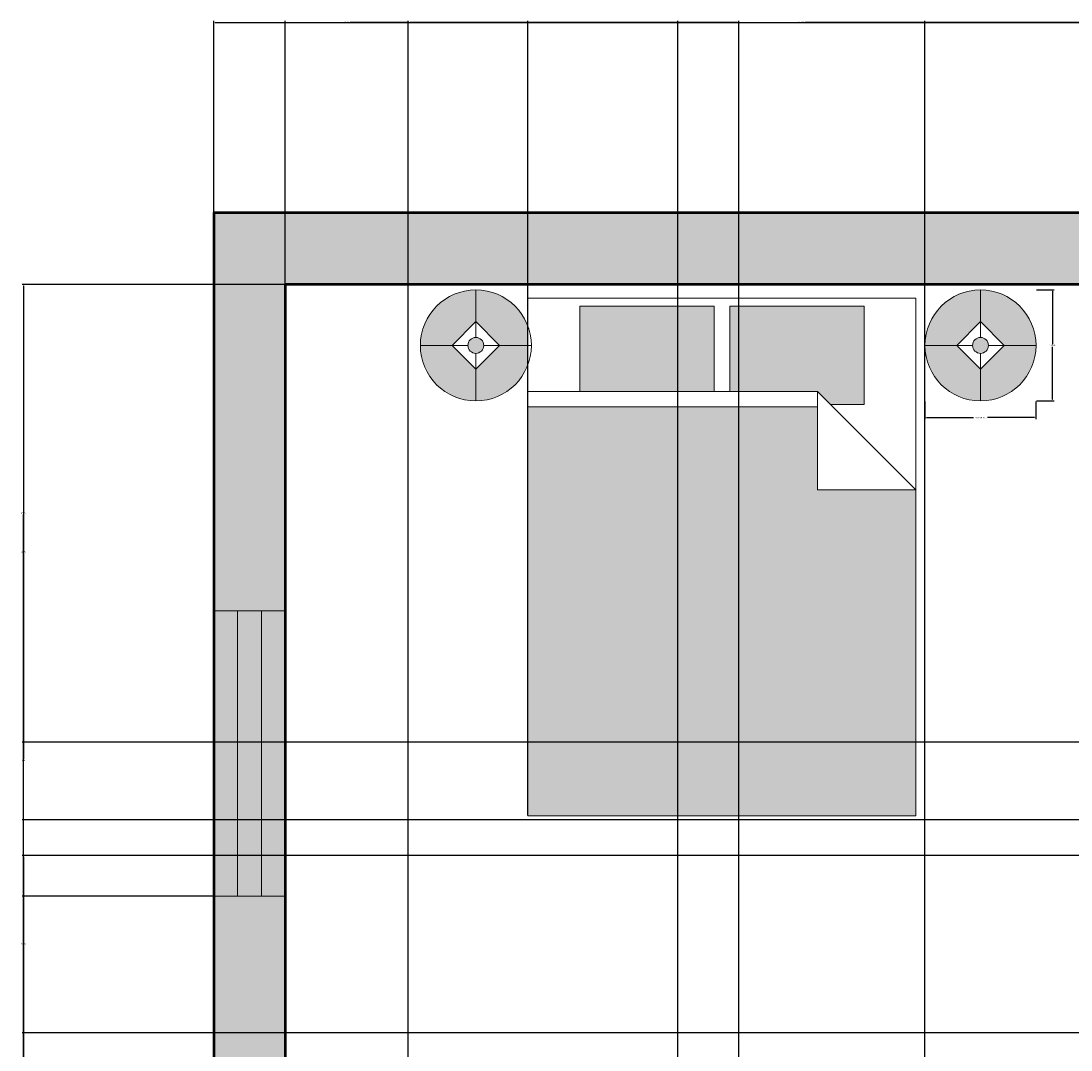
# Model space of a CAD drawing. Units: inches. Extents: x 1201 to 1754, y 247 to 775.
# Tile 7 of 10: x 1222 to 1355, y 645 to 775. Entities that reach past the tile are written whole.
import ezdxf

# ---------------------------------------------------------------- set-up
doc = ezdxf.new("R2010")
doc.units = ezdxf.units.IN
for name, color, linetype, lineweight in [('A-ANNO-DIMS', 2, 'Continuous', 18), ('A-FURN', 8, 'Continuous', 18), ('A-FURN-PATT', 9, 'Continuous', 13), ('A-GLAZ', 4, 'Continuous', 18), ('A-GLAZ-PATT', 9, 'Continuous', 13), ('A-WALL', 7, 'Continuous', 50), ('A-WALL-PATT', 9, 'Continuous', 13)]:
    doc.layers.add(name, color=color, linetype=linetype, lineweight=lineweight)
doc.styles.get("Standard").update_dxf_attribs({"font": 'arial.ttf'})
doc.dimstyles.get("Standard").update_dxf_attribs({"dimtxt": 0.18, "dimasz": 0.18, "dimexe": 0.18, "dimexo": 0.0625, "dimgap": 0.09, "dimtad": 0, "dimtih": 1, "dimtoh": 1, "dimdec": 4, "dimzin": 0, "dimdsep": 46, "dimtxsty": 'Standard', "dimcen": 0.09, "dimadec": 0, "dimazin": 0, "dimtfac": 1, "dimtdec": 4, "dimtofl": 0, "dimtmove": 0, "dimatfit": 3, "dimfxl": 1, "dimtolj": 1, "dimtzin": 0, "dimarcsym": 0})

# ---------------------------------------------------------------- blocks, each defined once
blk = doc.blocks.new('Bed - Queen')
for p, q in [((0, -80.00003), (0, 0)), ((0, 0), (59.99999, 0)), ((59.99999, 0), (59.99999, -80.00003)), ((7.99999, -1.2), (28.79998, -1.2)), ((7.99999, -14.4), (7.99999, -1.2)), ((28.79998, -1.2), (28.79998, -14.4)), ((31.19999, -1.2), (51.99999, -1.2)), ((31.19999, -14.4), (31.19999, -1.2)), ((51.99999, -1.2), (51.99999, -16.4)), ((0, -14.4), (44.8, -14.4)), ((59.99999, -29.6), (44.8, -14.4)), ((44.8, -14.4), (44.8, -29.6)), ((44.8, -16.8), (0, -16.8)), ((51.99999, -16.4), (46.79936, -16.4)), ((44.8, -29.6), (59.99999, -29.6)), ((59.99999, -80.00003), (0, -80.00003))]:
    blk.add_line(p, q)
blk = doc.blocks.new('Lamp - Table')
for p, q in [((0, 7), (0, 1)), ((0, 3), (-3, 0)), ((3, 0), (0, 3)), ((-1, 0), (-7, 0)), ((-3, 0), (0, -3)), ((0, -3), (3, 0)), ((1, 0), (7, 0)), ((0, -1), (0, -7))]:
    blk.add_line(p, q)
for radius in [7, 1]:
    blk.add_circle((0, 0), radius)
blk = doc.blocks.new('WIN-36IN-PLAN')
for p, q in [((9, 36), (0, 36)), ((3, 0), (3, 36)), ((6, 0), (6, 36))]:
    blk.add_line(p, q)
blk.add_lwpolyline([(0, 36), (0, 0), (9, 0), (9, 36)])
blk = doc.blocks.new('*D21')
at = {"layer": 'A-ANNO-DIMS', "color": 0, "lineweight": -2, "transparency": 16777216}
for p, q in [((1336.21, 727.18), (1336.21, 724.96)), ((1350.21, 727.18), (1350.21, 724.96)), ((1336.39, 725.14), (1342.31, 725.14)), ((1350.03, 725.14), (1344.11, 725.14))]:
    blk.add_line(p, q, dxfattribs=at)
at = {"layer": 'A-ANNO-DIMS', "color": 0, "transparency": 16777216}
for points in [[(1336.39, 725.17), (1336.39, 725.11), (1336.21, 725.14)], [(1350.03, 725.17), (1350.03, 725.11), (1350.21, 725.14)]]:
    blk.add_solid(points, dxfattribs=at)
at = {"layer": 'Defpoints', "color": 0, "transparency": 16777216}
for p in [(1336.21, 727.24), (1350.21, 727.24), (1350.21, 725.14)]:
    blk.add_point(p, dxfattribs=at)
at = {"layer": 'A-ANNO-DIMS', "color": 0, "transparency": 16777216, "insert": (1343.21, 725.14), "char_height": 0.18, "attachment_point": 5}
blk.add_mtext('\\A1;LAMP 14 TYP.', dxfattribs=at)
blk = doc.blocks.new('*D22')
at = {"layer": 'A-ANNO-DIMS', "color": 0, "lineweight": -2, "transparency": 16777216}
for p, q in [((1350.27, 741.24), (1352.49, 741.24)), ((1352.31, 741.06), (1352.31, 734.42)), ((1352.31, 727.42), (1352.31, 734.06)), ((1350.27, 727.24), (1352.49, 727.24))]:
    blk.add_line(p, q, dxfattribs=at)
at = {"layer": 'A-ANNO-DIMS', "color": 0, "transparency": 16777216}
for points in [[(1352.28, 741.06), (1352.34, 741.06), (1352.31, 741.24)], [(1352.28, 727.42), (1352.34, 727.42), (1352.31, 727.24)]]:
    blk.add_solid(points, dxfattribs=at)
at = {"layer": 'Defpoints', "color": 0, "transparency": 16777216}
for p in [(1350.21, 741.24), (1352.31, 741.24), (1350.21, 727.24)]:
    blk.add_point(p, dxfattribs=at)
at = {"layer": 'A-ANNO-DIMS', "color": 0, "transparency": 16777216, "insert": (1352.31, 734.24), "char_height": 0.18, "attachment_point": 5}
blk.add_mtext('\\A1;14 TYP.', dxfattribs=at)
blk = doc.blocks.new('*D45')
at = {"layer": 'A-ANNO-DIMS', "color": 0, "lineweight": -2, "transparency": 16777216}
for p, q in [((1246.52, 751), (1246.52, 775.14)), ((1246.7, 774.96), (1486.23, 774.96)), ((1726.34, 774.96), (1486.81, 774.96)), ((1726.52, 751), (1726.52, 775.14))]:
    blk.add_line(p, q, dxfattribs=at)
at = {"layer": 'A-ANNO-DIMS', "color": 0, "transparency": 16777216}
for points in [[(1246.7, 774.99), (1246.7, 774.93), (1246.52, 774.96)], [(1726.34, 774.99), (1726.34, 774.93), (1726.52, 774.96)]]:
    blk.add_solid(points, dxfattribs=at)
at = {"layer": 'Defpoints', "color": 0, "transparency": 16777216}
for p in [(1726.52, 774.96), (1246.52, 750.94), (1726.52, 750.94)]:
    blk.add_point(p, dxfattribs=at)
at = {"layer": 'A-ANNO-DIMS', "color": 0, "transparency": 16777216, "insert": (1486.52, 774.96), "char_height": 0.18, "attachment_point": 5}
blk.add_mtext('\\A1;480', dxfattribs=at)
blk = doc.blocks.new('*D47')
at = {"layer": 'A-ANNO-DIMS', "color": 0, "lineweight": -2, "transparency": 16777216}
for p, q in [((1255.52, 742), (1255.52, 775.14)), ((1255.7, 774.96), (1363.23, 774.96)), ((1471.34, 774.96), (1363.81, 774.96)), ((1471.52, 742), (1471.52, 775.14))]:
    blk.add_line(p, q, dxfattribs=at)
at = {"layer": 'A-ANNO-DIMS', "color": 0, "transparency": 16777216}
for points in [[(1255.7, 774.99), (1255.7, 774.93), (1255.52, 774.96)], [(1471.34, 774.99), (1471.34, 774.93), (1471.52, 774.96)]]:
    blk.add_solid(points, dxfattribs=at)
at = {"layer": 'Defpoints', "color": 0, "transparency": 16777216}
for p in [(1471.52, 774.96), (1255.52, 741.94), (1471.52, 741.94)]:
    blk.add_point(p, dxfattribs=at)
at = {"layer": 'A-ANNO-DIMS', "color": 0, "transparency": 16777216, "insert": (1363.52, 774.96), "char_height": 0.18, "attachment_point": 5}
blk.add_mtext('\\A1;216', dxfattribs=at)
blk = doc.blocks.new('*D48')
at = {"layer": 'A-ANNO-DIMS', "color": 0, "lineweight": -2, "transparency": 16777216}
for p, q in [((1255.46, 741.94), (1222.33, 741.94)), ((1222.51, 741.76), (1222.51, 682.12)), ((1222.51, 622.12), (1222.51, 681.76)), ((1255.46, 621.94), (1222.33, 621.94))]:
    blk.add_line(p, q, dxfattribs=at)
at = {"layer": 'A-ANNO-DIMS', "color": 0, "transparency": 16777216}
for points in [[(1222.48, 741.76), (1222.54, 741.76), (1222.51, 741.94)], [(1222.48, 622.12), (1222.54, 622.12), (1222.51, 621.94)]]:
    blk.add_solid(points, dxfattribs=at)
at = {"layer": 'Defpoints', "color": 0, "transparency": 16777216}
for p in [(1222.51, 741.94), (1255.52, 741.94), (1255.52, 621.94)]:
    blk.add_point(p, dxfattribs=at)
at = {"layer": 'A-ANNO-DIMS', "color": 0, "transparency": 16777216, "insert": (1222.51, 681.94), "char_height": 0.18, "attachment_point": 5}
blk.add_mtext('\\A1;120', dxfattribs=at)
blk = doc.blocks.new('*D52')
at = {"layer": 'A-ANNO-DIMS', "color": 0, "lineweight": -2, "transparency": 16777216}
for p, q in [((1477.46, 669.94), (1222.33, 669.94)), ((1222.51, 669.76), (1222.51, 616.12)), ((1222.51, 562.12), (1222.51, 615.76)), ((1477.46, 561.94), (1222.33, 561.94))]:
    blk.add_line(p, q, dxfattribs=at)
at = {"layer": 'A-ANNO-DIMS', "color": 0, "transparency": 16777216}
for points in [[(1222.48, 669.76), (1222.54, 669.76), (1222.51, 669.94)], [(1222.48, 562.12), (1222.54, 562.12), (1222.51, 561.94)]]:
    blk.add_solid(points, dxfattribs=at)
at = {"layer": 'Defpoints', "color": 0, "transparency": 16777216}
for p in [(1222.51, 669.94), (1477.52, 669.94), (1477.52, 561.94)]:
    blk.add_point(p, dxfattribs=at)
at = {"layer": 'A-ANNO-DIMS', "color": 0, "transparency": 16777216, "insert": (1222.51, 615.94), "char_height": 0.18, "attachment_point": 5}
blk.add_mtext('\\A1;108', dxfattribs=at)
blk = doc.blocks.new('*D53')
at = {"layer": 'A-ANNO-DIMS', "color": 0, "lineweight": -2, "transparency": 16777216}
for p, q in [((1717.46, 741.94), (1222.33, 741.94)), ((1222.51, 741.76), (1222.51, 708.37)), ((1222.51, 674.62), (1222.51, 708.01)), ((1657.46, 674.44), (1222.33, 674.44))]:
    blk.add_line(p, q, dxfattribs=at)
at = {"layer": 'A-ANNO-DIMS', "color": 0, "transparency": 16777216}
for points in [[(1222.48, 741.76), (1222.54, 741.76), (1222.51, 741.94)], [(1222.48, 674.62), (1222.54, 674.62), (1222.51, 674.44)]]:
    blk.add_solid(points, dxfattribs=at)
at = {"layer": 'Defpoints', "color": 0, "transparency": 16777216}
for p in [(1222.51, 741.94), (1717.52, 741.94), (1657.52, 674.44)]:
    blk.add_point(p, dxfattribs=at)
at = {"layer": 'A-ANNO-DIMS', "color": 0, "transparency": 16777216, "insert": (1222.51, 708.19), "char_height": 0.18, "attachment_point": 5}
blk.add_mtext('\\A1;67.5', dxfattribs=at)
blk = doc.blocks.new('*D54')
at = {"layer": 'A-ANNO-DIMS', "color": 0, "lineweight": -2, "transparency": 16777216}
for p, q in [((1255.52, 562), (1255.52, 775.14)), ((1255.7, 774.96), (1324.88, 774.96)), ((1394.84, 774.96), (1325.66, 774.96)), ((1395.02, 562), (1395.02, 775.14))]:
    blk.add_line(p, q, dxfattribs=at)
at = {"layer": 'A-ANNO-DIMS', "color": 0, "transparency": 16777216}
for points in [[(1255.7, 774.99), (1255.7, 774.93), (1255.52, 774.96)], [(1394.84, 774.99), (1394.84, 774.93), (1395.02, 774.96)]]:
    blk.add_solid(points, dxfattribs=at)
at = {"layer": 'Defpoints', "color": 0, "transparency": 16777216}
for p in [(1395.02, 774.96), (1255.52, 561.94), (1395.02, 561.94)]:
    blk.add_point(p, dxfattribs=at)
at = {"layer": 'A-ANNO-DIMS', "color": 0, "transparency": 16777216, "insert": (1325.27, 774.96), "char_height": 0.18, "attachment_point": 5}
blk.add_mtext('\\A1;139.5', dxfattribs=at)
blk = doc.blocks.new('*D59')
at = {"layer": 'A-ANNO-DIMS', "color": 0, "lineweight": -2, "transparency": 16777216}
for p, q in [((1255.52, 418), (1255.52, 775.14)), ((1255.7, 774.96), (1330.24, 774.96)), ((1405.34, 774.96), (1330.8, 774.96)), ((1405.52, 418), (1405.52, 775.14))]:
    blk.add_line(p, q, dxfattribs=at)
at = {"layer": 'A-ANNO-DIMS', "color": 0, "transparency": 16777216}
for points in [[(1255.7, 774.99), (1255.7, 774.93), (1255.52, 774.96)], [(1405.34, 774.99), (1405.34, 774.93), (1405.52, 774.96)]]:
    blk.add_solid(points, dxfattribs=at)
at = {"layer": 'Defpoints', "color": 0, "transparency": 16777216}
for p in [(1405.52, 774.96), (1255.52, 417.94), (1405.52, 417.94)]:
    blk.add_point(p, dxfattribs=at)
at = {"layer": 'A-ANNO-DIMS', "color": 0, "transparency": 16777216, "insert": (1330.52, 774.96), "char_height": 0.18, "attachment_point": 5}
blk.add_mtext('\\A1;150', dxfattribs=at)
blk = doc.blocks.new('*D73')
at = {"layer": 'A-ANNO-DIMS', "color": 0, "lineweight": -2, "transparency": 16777216}
for p, q in [((1246.46, 664.8), (1222.33, 664.8)), ((1222.51, 664.62), (1222.51, 630.52)), ((1222.51, 596.07), (1222.51, 630.16)), ((1246.46, 595.89), (1222.33, 595.89))]:
    blk.add_line(p, q, dxfattribs=at)
at = {"layer": 'A-ANNO-DIMS', "color": 0, "transparency": 16777216}
for points in [[(1222.48, 664.62), (1222.54, 664.62), (1222.51, 664.8)], [(1222.48, 596.07), (1222.54, 596.07), (1222.51, 595.89)]]:
    blk.add_solid(points, dxfattribs=at)
at = {"layer": 'Defpoints', "color": 0, "transparency": 16777216}
for p in [(1222.51, 664.8), (1246.52, 664.8), (1246.52, 595.89)]:
    blk.add_point(p, dxfattribs=at)
at = {"layer": 'A-ANNO-DIMS', "color": 0, "transparency": 16777216, "insert": (1222.51, 630.34), "char_height": 0.18, "attachment_point": 5}
blk.add_mtext('\\A1;68.91', dxfattribs=at)
blk = doc.blocks.new('*D76')
at = {"layer": 'A-ANNO-DIMS', "color": 0, "lineweight": -2, "transparency": 16777216}
for p, q in [((1717.46, 669.94), (1222.33, 669.94)), ((1222.51, 669.76), (1222.51, 658.95)), ((1222.51, 647.78), (1222.51, 658.59)), ((1717.46, 647.6), (1222.33, 647.6))]:
    blk.add_line(p, q, dxfattribs=at)
at = {"layer": 'A-ANNO-DIMS', "color": 0, "transparency": 16777216}
for points in [[(1222.48, 669.76), (1222.54, 669.76), (1222.51, 669.94)], [(1222.48, 647.78), (1222.54, 647.78), (1222.51, 647.6)]]:
    blk.add_solid(points, dxfattribs=at)
at = {"layer": 'Defpoints', "color": 0, "transparency": 16777216}
for p in [(1222.51, 669.94), (1717.52, 669.94), (1717.52, 647.6)]:
    blk.add_point(p, dxfattribs=at)
at = {"layer": 'A-ANNO-DIMS', "color": 0, "transparency": 16777216, "insert": (1222.51, 658.77), "char_height": 0.18, "attachment_point": 5}
blk.add_mtext('\\A1;22.34', dxfattribs=at)
blk = doc.blocks.new('*D85')
at = {"layer": 'A-ANNO-DIMS', "color": 0, "lineweight": -2, "transparency": 16777216}
for p, q in [((1255.52, 629.73), (1255.52, 775.14)), ((1255.7, 774.96), (1283.75, 774.96)), ((1312.55, 774.96), (1284.5, 774.96)), ((1312.73, 629.73), (1312.73, 775.14))]:
    blk.add_line(p, q, dxfattribs=at)
at = {"layer": 'A-ANNO-DIMS', "color": 0, "transparency": 16777216}
for points in [[(1255.7, 774.99), (1255.7, 774.93), (1255.52, 774.96)], [(1312.55, 774.99), (1312.55, 774.93), (1312.73, 774.96)]]:
    blk.add_solid(points, dxfattribs=at)
at = {"layer": 'Defpoints', "color": 0, "transparency": 16777216}
for p in [(1312.73, 774.96), (1255.52, 629.66), (1312.73, 629.66)]:
    blk.add_point(p, dxfattribs=at)
at = {"layer": 'A-ANNO-DIMS', "color": 0, "transparency": 16777216, "insert": (1284.13, 774.96), "char_height": 0.18, "attachment_point": 5}
blk.add_mtext('\\A1;57.21', dxfattribs=at)
blk = doc.blocks.new('*D87')
at = {"layer": 'A-ANNO-DIMS', "color": 0, "lineweight": -2, "transparency": 16777216}
for p, q in [((1459.84, 741.94), (1222.33, 741.94)), ((1222.51, 741.76), (1222.51, 713.27)), ((1222.51, 684.41), (1222.51, 712.91)), ((1459.84, 684.23), (1222.33, 684.23))]:
    blk.add_line(p, q, dxfattribs=at)
at = {"layer": 'A-ANNO-DIMS', "color": 0, "transparency": 16777216}
for points in [[(1222.48, 741.76), (1222.54, 741.76), (1222.51, 741.94)], [(1222.48, 684.41), (1222.54, 684.41), (1222.51, 684.23)]]:
    blk.add_solid(points, dxfattribs=at)
at = {"layer": 'Defpoints', "color": 0, "transparency": 16777216}
for p in [(1222.51, 741.94), (1459.9, 741.94), (1459.9, 684.23)]:
    blk.add_point(p, dxfattribs=at)
at = {"layer": 'A-ANNO-DIMS', "color": 0, "transparency": 16777216, "insert": (1222.51, 713.09), "char_height": 0.18, "attachment_point": 5}
blk.add_mtext('\\A1;57.71', dxfattribs=at)
blk = doc.blocks.new('*D91')
at = {"layer": 'A-ANNO-DIMS', "color": 0, "lineweight": -2, "transparency": 16777216}
for p, q in [((1255.52, 664.86), (1255.52, 775.14)), ((1255.7, 774.96), (1270.37, 774.96)), ((1285.96, 774.96), (1271.29, 774.96)), ((1286.14, 675.01), (1286.14, 775.14))]:
    blk.add_line(p, q, dxfattribs=at)
at = {"layer": 'A-ANNO-DIMS', "color": 0, "transparency": 16777216}
for points in [[(1255.7, 774.99), (1255.7, 774.93), (1255.52, 774.96)], [(1285.96, 774.99), (1285.96, 774.93), (1286.14, 774.96)]]:
    blk.add_solid(points, dxfattribs=at)
at = {"layer": 'Defpoints', "color": 0, "transparency": 16777216}
for p in [(1286.14, 774.96), (1286.14, 674.95), (1255.52, 664.8)]:
    blk.add_point(p, dxfattribs=at)
at = {"layer": 'A-ANNO-DIMS', "color": 0, "transparency": 16777216, "insert": (1270.83, 774.96), "char_height": 0.18, "attachment_point": 5}
blk.add_mtext('\\A1;30.617', dxfattribs=at)
blk = doc.blocks.new('*D94')
at = {"layer": 'A-ANNO-DIMS', "color": 0, "lineweight": -2, "transparency": 16777216}
for p, q in [((1305.02, 443.29), (1305.02, 775.14)), ((1305.2, 774.96), (1320.15, 774.96)), ((1336.03, 774.96), (1321.08, 774.96)), ((1336.21, 449.65), (1336.21, 775.14))]:
    blk.add_line(p, q, dxfattribs=at)
at = {"layer": 'A-ANNO-DIMS', "color": 0, "transparency": 16777216}
for points in [[(1305.2, 774.99), (1305.2, 774.93), (1305.02, 774.96)], [(1336.03, 774.99), (1336.03, 774.93), (1336.21, 774.96)]]:
    blk.add_solid(points, dxfattribs=at)
at = {"layer": 'Defpoints', "color": 0, "transparency": 16777216}
for p in [(1336.21, 774.96), (1336.21, 449.58), (1305.02, 443.23)]:
    blk.add_point(p, dxfattribs=at)
at = {"layer": 'A-ANNO-DIMS', "color": 0, "transparency": 16777216, "insert": (1320.61, 774.96), "char_height": 0.18, "attachment_point": 5}
blk.add_mtext('\\A1;31.195', dxfattribs=at)
blk = doc.blocks.new('*D97')
at = {"layer": 'A-ANNO-DIMS', "color": 0, "lineweight": -2, "transparency": 16777216}
for p, q in [((1255.52, 506.76), (1255.52, 775.14)), ((1255.7, 774.96), (1262.81, 774.96)), ((1270.84, 774.96), (1263.72, 774.96)), ((1271.02, 485.29), (1271.02, 775.14))]:
    blk.add_line(p, q, dxfattribs=at)
at = {"layer": 'A-ANNO-DIMS', "color": 0, "transparency": 16777216}
for points in [[(1255.7, 774.99), (1255.7, 774.93), (1255.52, 774.96)], [(1270.84, 774.99), (1270.84, 774.93), (1271.02, 774.96)]]:
    blk.add_solid(points, dxfattribs=at)
at = {"layer": 'Defpoints', "color": 0, "transparency": 16777216}
for p in [(1271.02, 774.96), (1255.52, 506.7), (1271.02, 485.23)]:
    blk.add_point(p, dxfattribs=at)
at = {"layer": 'A-ANNO-DIMS', "color": 0, "transparency": 16777216, "insert": (1263.27, 774.96), "char_height": 0.18, "attachment_point": 5}
blk.add_mtext('\\A1;15.496', dxfattribs=at)

msp = doc.modelspace()

# ---------------------------------------------------------------- hatches: boundary and pattern name
at = {"layer": 'A-FURN-PATT'}
h = msp.add_hatch(color=256, dxfattribs=at)
h.dxf.hatch_style = 1
h.paths.add_polyline_path([(1335.0621, 716.0469), (1322.6678, 716.0469), (1322.6678, 726.4842), (1286.1373, 726.4842), (1286.1373, 674.95), (1335.0621, 674.95)])
h.paths.add_polyline_path([(1328.5388, 739.2047), (1311.5782, 739.2047), (1311.5782, 728.4412), (1322.6678, 728.4412), (1324.2987, 726.8104), (1328.5388, 726.8104)])
h.paths.add_polyline_path([(1309.6212, 739.2047), (1292.6606, 739.2047), (1292.6606, 728.4412), (1309.6212, 728.4412)])
h.paths.add_polyline_path([(1346.7317, 603.3316), (1338.7317, 603.3316, 0.48007965), (1341.0876, 585.8086, 0.21500378), (1344.3757, 585.8086, 0.4800795)])
h.paths.add_polyline_path([(1315.398, 617.4415), (1255.5208, 617.4415), (1255.5208, 581.4415), (1315.398, 581.4415)])
h.paths.add_polyline_path([(1297.398, 585.4415), (1261.398, 585.4415, -0.50000012), (1259.398, 587.4415), (1259.398, 611.4415, -0.50000012), (1261.398, 613.4415), (1297.398, 613.4415, -1)], flags=16)
h.paths.add_polyline_path([(1262.898, 599.4415, -1), (1265.898, 599.4415, -1)], flags=0)
h.paths.add_polyline_path([(1263.398, 599.4415, -1), (1265.398, 599.4415, -1)], flags=0)
h.paths.add_polyline_path([(1352.2316, 615.3316, 0.50000012), (1351.2316, 616.3316), (1334.2316, 616.3316, 0.50000012), (1333.2316, 615.3316), (1333.2316, 611.3316, 0.50000012), (1334.2316, 610.3316), (1351.2316, 610.3316, 0.50000012), (1352.2316, 611.3316)])
h.paths.add_polyline_path([(1335.7316, 609.3316), (1334.7316, 609.3316), (1334.7316, 608.8316), (1332.7316, 608.8316), (1332.7316, 607.8316), (1335.7316, 607.8316)])
h.paths.add_polyline_path([(1537.5652, 741.6115), (1477.5652, 741.6115), (1477.5652, 705.6115), (1537.5652, 705.6115)])
h.paths.add_polyline_path([(1519.5652, 709.6115), (1483.5652, 709.6115, -0.50000012), (1481.5652, 711.6115), (1481.5652, 735.6115, -0.50000012), (1483.5652, 737.6115), (1519.5652, 737.6115, -1)], flags=16)
h.paths.add_polyline_path([(1485.0652, 723.6115, -1), (1488.0652, 723.6115, -1)], flags=0)
h.paths.add_polyline_path([(1485.5652, 723.6115, -1), (1487.5652, 723.6115, -1)], flags=0)
h.paths.add_polyline_path([(1712.1885, 727.9922), (1704.1885, 727.9922, 0.48007965), (1706.5444, 710.4693, 0.21500378), (1709.8325, 710.4693, 0.4800795)])
h.paths.add_polyline_path([(1701.1884, 733.9922), (1700.1884, 733.9922), (1700.1884, 733.4922), (1698.1884, 733.4922), (1698.1884, 732.4922), (1701.1884, 732.4922)])
h.paths.add_polyline_path([(1717.5208, 740.6473, 0.27397494), (1716.6884, 740.9922), (1699.6884, 740.9922, 0.50000012), (1698.6884, 739.9922), (1698.6884, 735.9922, 0.50000012), (1699.6884, 734.9922), (1716.6884, 734.9922, 0.27397494), (1717.5208, 735.3372)])
h.paths.add_polyline_path([(1586.346, 642.6772), (1573.9517, 642.6772), (1573.9517, 653.1145), (1537.4212, 653.1145), (1537.4212, 601.5803), (1586.346, 601.5803)])
h.paths.add_polyline_path([(1579.8227, 665.835), (1562.8621, 665.835), (1562.8621, 655.0715), (1573.9517, 655.0715), (1575.5826, 653.4407), (1579.8227, 653.4407)])
h.paths.add_polyline_path([(1560.9051, 665.835), (1543.9445, 665.835), (1543.9445, 655.0715), (1560.9051, 655.0715)])
h = msp.add_hatch(color=256, dxfattribs=at)
h.dxf.hatch_style = 1
h.paths.add_polyline_path([(1344.212, 734.2435, 1), (1342.212, 734.2435, 1)])
h.paths.add_polyline_path([(1343.212, 741.2435), (1343.212, 737.2435), (1346.212, 734.2435), (1350.212, 734.2435, 0.41421356)])
h.paths.add_polyline_path([(1350.212, 734.2435), (1346.212, 734.2435), (1343.212, 731.2435), (1343.212, 727.2435, 0.41421356)])
h.paths.add_polyline_path([(1343.212, 731.2435), (1340.212, 734.2435), (1336.212, 734.2435, 0.41421356), (1343.212, 727.2435)])
h.paths.add_polyline_path([(1343.212, 737.2435), (1343.212, 741.2435, 0.41421356), (1336.212, 734.2435), (1340.212, 734.2435)])
h.paths.add_polyline_path([(1286.1373, 731.8347), (1286.1373, 734.2435), (1282.5648, 734.2435), (1279.5648, 731.2435), (1279.5648, 727.2435, 0.31468394)])
h.paths.add_polyline_path([(1276.5648, 734.2435), (1272.5648, 734.2435, 0.41421356), (1279.5648, 727.2435), (1279.5648, 731.2435)])
h.paths.add_polyline_path([(1279.5648, 741.2435, 0.41421356), (1272.5648, 734.2435), (1276.5648, 734.2435), (1279.5648, 737.2435)])
h.paths.add_polyline_path([(1286.1373, 736.6524, 0.31468394), (1279.5648, 741.2435), (1279.5648, 737.2435), (1282.5648, 734.2435), (1286.1373, 734.2435)])
h.paths.add_polyline_path([(1278.5648, 734.2435, 1), (1280.5648, 734.2435, 1)])
h.paths.add_polyline_path([(1594.9356, 658.7794), (1591.9356, 661.7794), (1587.9356, 661.7794, 0.41421356), (1594.9356, 654.7794)])
h.paths.add_polyline_path([(1601.9356, 661.7794), (1597.9356, 661.7794), (1594.9356, 658.7794), (1594.9356, 654.7794, 0.41421356)])
h.paths.add_polyline_path([(1594.9356, 668.7794), (1594.9356, 664.7794), (1597.9356, 661.7794), (1601.9356, 661.7794, 0.41421356)])
h.paths.add_polyline_path([(1594.9356, 664.7794), (1594.9356, 668.7794, 0.41421356), (1587.9356, 661.7794), (1591.9356, 661.7794)])
h.paths.add_polyline_path([(1593.9356, 661.7794, 1), (1595.9356, 661.7794, 1)])
h.paths.add_polyline_path([(1528.896, 661.4743, 1), (1526.896, 661.4743, 1)])
h.paths.add_polyline_path([(1527.896, 668.4743), (1527.896, 664.4743), (1530.896, 661.4743), (1534.896, 661.4743, 0.41421356)])
h.paths.add_polyline_path([(1534.896, 661.4743), (1530.896, 661.4743), (1527.896, 658.4743), (1527.896, 654.4743, 0.41421356)])
h.paths.add_polyline_path([(1524.896, 661.4743), (1520.896, 661.4743, 0.41421356), (1527.896, 654.4743), (1527.896, 658.4743)])
h.paths.add_polyline_path([(1527.896, 668.4743, 0.41421356), (1520.896, 661.4743), (1524.896, 661.4743), (1527.896, 664.4743)])
at = {"layer": 'A-GLAZ-PATT'}
h = msp.add_hatch(color=256, dxfattribs=at)
h.dxf.hatch_style = 1
h.set_gradient(color1=(0, 0, 255), color2=(255, 255, 0), name='SPHERICAL')
h.paths.add_polyline_path([(1252.5208, 700.7954), (1249.5208, 700.7954), (1249.5208, 664.7954), (1252.5208, 664.7954)])
h.paths.add_polyline_path([(1249.5208, 700.7954), (1246.5208, 700.7954), (1246.5208, 664.7954), (1249.5208, 664.7954)])
h.paths.add_polyline_path([(1255.5208, 700.7954), (1252.5208, 700.7954), (1252.5208, 664.7954), (1255.5208, 664.7954)])
at = {"layer": 'A-WALL-PATT'}
h = msp.add_hatch(color=256, dxfattribs=at)
h.dxf.hatch_style = 1
h.paths.add_polyline_path([(1255.5208, 741.9415), (1471.5208, 741.9415), (1471.5208, 684.2327), (1471.5208, 602.9415), (1477.5208, 602.9415), (1477.5208, 669.9415), (1618.5208, 669.9415), (1618.5208, 674.4415), (1477.5208, 674.4415), (1477.5208, 741.9415), (1481.2969, 741.9415), (1481.2969, 750.9415), (1246.5208, 750.9415), (1246.5208, 700.7954), (1255.5208, 700.7954)])
h.paths.add_polyline_path([(1255.5208, 557.4415), (1399.5208, 557.4415), (1399.5208, 617.4415), (1423.5208, 617.4415), (1423.5208, 621.9415), (1392.0208, 621.9415), (1392.0208, 617.4415), (1395.0208, 617.4415), (1395.0208, 561.9415), (1255.5208, 561.9415), (1255.5208, 571.8878), (1246.5208, 571.8878), (1246.5208, 506.6967), (1255.5208, 506.6967)])
h.paths.add_polyline_path([(1255.5208, 664.7954), (1246.5208, 664.7954), (1246.5208, 595.8878), (1255.398, 595.8878), (1255.398, 617.4415), (1315.398, 617.4415), (1356.0208, 617.4415), (1356.0208, 618.0127), (1356.0208, 621.9415), (1255.5208, 621.9415), (1255.5208, 629.6628)])
h.paths.add_polyline_path([(1255.5208, 470.6967), (1246.5208, 470.6967), (1246.5208, 347.7487), (1255.5208, 347.7487), (1255.5208, 413.4415), (1405.5208, 413.4415), (1405.5208, 417.9415), (1255.5208, 417.9415)])
h.paths.add_polyline_path([(1290.9481, 279.9415), (1255.5208, 279.9415), (1255.5208, 311.7487), (1246.5208, 311.7487), (1246.5208, 270.9415), (1290.9481, 270.9415)])
h.paths.add_polyline_path([(1486.5907, 279.9415), (1477.5208, 279.9415), (1477.5208, 417.9415), (1468.5208, 417.9415), (1468.5208, 413.4415), (1471.5208, 413.4415), (1471.5208, 279.9415), (1399.0105, 279.9415), (1399.0105, 270.9415), (1486.5907, 270.9415)])
h.paths.add_polyline_path([(1563.0208, 279.9415), (1542.0208, 279.9415), (1542.0208, 417.9415), (1501.5208, 417.9415), (1501.5208, 413.4415), (1513.81, 413.4415), (1513.8125, 413.6987), (1537.8114, 413.4623), (1537.5208, 383.9637), (1537.5208, 279.9415), (1522.5907, 279.9415), (1522.5907, 270.9415), (1563.0208, 270.9415)])
h.paths.add_polyline_path([(1726.5208, 404.0342), (1717.5208, 404.0342), (1717.5208, 279.9415), (1641.0208, 279.9415), (1641.0208, 270.9415), (1726.5208, 270.9415)])
h.paths.add_polyline_path([(1726.5208, 507.4363), (1717.5208, 507.4363), (1717.5208, 440.0342), (1726.5208, 440.0342)])
h.paths.add_polyline_path([(1726.5208, 611.6009), (1717.5208, 611.6009), (1717.5208, 561.9415), (1477.5208, 561.9415), (1471.5208, 561.9692), (1471.5208, 557.4415), (1717.5208, 557.4415), (1717.5208, 543.4363), (1726.5208, 543.4363)])
h.paths.add_polyline_path([(1726.5208, 750.9415), (1505.2969, 750.9415), (1505.2969, 741.9415), (1697.6884, 741.9415), (1697.6884, 741.9922), (1718.6884, 741.9922), (1718.6884, 733.9922), (1717.5208, 733.9922), (1717.5208, 674.4415), (1660.5208, 674.4415), (1660.5208, 669.9415), (1717.5208, 669.9415), (1717.5208, 647.6009), (1726.5208, 647.6009)])

# ---------------------------------------------------------------- linework, layer by layer
at = {"layer": 'A-WALL'}
for p, q in [((1255.5208, 741.9415), (1255.5208, 621.9415)), ((1471.5208, 741.9415), (1255.5208, 741.9415))]:
    msp.add_line(p, q, dxfattribs=at)
msp.add_lwpolyline([(1638.0208, 270.9415), (1726.5208, 270.9415), (1726.5208, 750.9415), (1246.5208, 750.9415), (1246.5208, 270.9415), (1566.0208, 270.9415)], dxfattribs=at)

# ---------------------------------------------------------------- block references
at = {"layer": 'A-FURN'}
for p in [(1279.5648, 734.2435), (1343.212, 734.2435)]:
    msp.add_blockref('Lamp - Table', p, dxfattribs=at)
at = {"layer": 'A-FURN', "xscale": 0.8154145585976698, "yscale": 0.8154145585976698, "zscale": 0.8154145585976698}
msp.add_blockref('Bed - Queen', (1286.1373, 740.1832), dxfattribs=at)
at = {"layer": 'A-GLAZ'}
msp.add_blockref('WIN-36IN-PLAN', (1246.5208, 664.7954), dxfattribs=at)

# ---------------------------------------------------------------- dimensions: what is measured, and where the dimension line sits
at = {"layer": 'A-ANNO-DIMS'}
for base, p1, p2, override, picture, middle in [((1726.5208, 774.9565), (1246.5208, 750.9415), (1726.5208, 750.9415), {"dimdec": 0, "dimlfac": 1, "dimrnd": 0, "dimzin": 0, "dimdsep": 46, "dimlunit": 2}, '*D45', (1486.5208, 774.9565)), ((1471.5208, 774.9565), (1255.5208, 741.9415), (1471.5208, 741.9415), {"dimdec": 0, "dimlfac": 1, "dimrnd": 0, "dimzin": 0, "dimdsep": 46, "dimlunit": 2}, '*D47', (1363.5208, 774.9565)), ((1395.0208, 774.9565), (1255.5208, 561.9415), (1395.0208, 561.9415), {"dimdec": 1, "dimlfac": 1, "dimrnd": 0, "dimzin": 0, "dimdsep": 46, "dimlunit": 2}, '*D54', (1325.2708, 774.9565)), ((1405.5208, 774.9565), (1255.5208, 417.9415), (1405.5208, 417.9415), {"dimdec": 0, "dimlfac": 1, "dimrnd": 0, "dimzin": 0, "dimdsep": 46, "dimlunit": 2}, '*D59', (1330.5208, 774.9565)), ((1312.7334, 774.9565), (1255.5208, 629.6628), (1312.7334, 629.6628), {"dimdec": 2, "dimlfac": 1, "dimrnd": 0, "dimzin": 0, "dimdsep": 46, "dimlunit": 2}, '*D85', (1284.1271, 774.9565)), ((1286.13728, 774.95647), (1255.52076, 664.79541), (1286.13728, 674.95002), {"dimdec": 3, "dimlfac": 1, "dimrnd": 0, "dimzin": 0, "dimdsep": 46, "dimlunit": 2}, '*D91', (1270.82902, 774.95647)), ((1271.0165, 774.9565), (1255.5208, 506.6967), (1271.0165, 485.2267), {"dimdec": 3, "dimlfac": 1, "dimrnd": 0, "dimzin": 0, "dimdsep": 46, "dimlunit": 2}, '*D97', (1263.2686, 774.9565)), ((1336.2113, 774.9565), (1305.0165, 443.2267), (1336.2113, 449.5839), {"dimdec": 3, "dimlfac": 1, "dimrnd": 0, "dimzin": 0, "dimdsep": 46, "dimlunit": 2}, '*D94', (1320.6139, 774.9565))]:
    dim = msp.add_linear_dim(base=base, p1=p1, p2=p2, dimstyle='Standard', override=override, dxfattribs=at)
    dim.commit()
    dim.dimension.update_dxf_attribs({"geometry": picture, "text_midpoint": middle})
for base, p1, p2, override, picture, middle in [((1222.5058, 741.9415), (1459.8979, 684.2327), (1459.8979, 741.9415), {"dimdec": 2, "dimlfac": 1, "dimrnd": 0, "dimzin": 0, "dimdsep": 46, "dimlunit": 2}, '*D87', (1222.5058, 713.0871)), ((1222.5058, 741.9415), (1657.5208, 674.4415), (1717.5208, 741.9415), {"dimdec": 1, "dimlfac": 1, "dimrnd": 0, "dimzin": 0, "dimdsep": 46, "dimlunit": 2}, '*D53', (1222.5058, 708.1915)), ((1222.5058, 741.9415), (1255.5208, 621.9415), (1255.5208, 741.9415), {"dimdec": 0, "dimlfac": 1, "dimrnd": 0, "dimzin": 0, "dimdsep": 46, "dimlunit": 2}, '*D48', (1222.5058, 681.9415)), ((1222.5058, 669.9415), (1717.5208, 647.6009), (1717.5208, 669.9415), {"dimdec": 2, "dimlfac": 1, "dimrnd": 0, "dimzin": 0, "dimdsep": 46, "dimlunit": 2}, '*D76', (1222.5058, 658.7712)), ((1222.5058, 669.9415), (1477.5208, 561.9415), (1477.5208, 669.9415), {"dimdec": 0, "dimlfac": 1, "dimrnd": 0, "dimzin": 0, "dimdsep": 46, "dimlunit": 2}, '*D52', (1222.5058, 615.9415)), ((1222.5058, 664.7954), (1246.5208, 595.8878), (1246.5208, 664.7954), {"dimdec": 2, "dimlfac": 1, "dimrnd": 0, "dimzin": 0, "dimdsep": 46, "dimlunit": 2}, '*D73', (1222.5058, 630.3416))]:
    dim = msp.add_linear_dim(base=base, p1=p1, p2=p2, angle=90, dimstyle='Standard', override=override, dxfattribs=at)
    dim.commit()
    dim.dimension.update_dxf_attribs({"geometry": picture, "text_midpoint": middle})
dim = msp.add_linear_dim(base=(1352.312, 741.2435), p1=(1350.212, 727.2435), p2=(1350.212, 741.2435), angle=90, text='<> TYP.', dimstyle='Standard', override={"dimdec": 0, "dimlfac": 1, "dimrnd": 0, "dimzin": 0, "dimdsep": 46, "dimlunit": 2}, dxfattribs=at)
dim.commit()
dim.dimension.update_dxf_attribs({"geometry": '*D22', "text_midpoint": (1352.312, 734.2435)})
dim = msp.add_linear_dim(base=(1350.212, 725.1435), p1=(1336.212, 727.2435), p2=(1350.212, 727.2435), text='LAMP <> TYP.', dimstyle='Standard', override={"dimdec": 0, "dimlfac": 1, "dimrnd": 0, "dimzin": 0, "dimdsep": 46, "dimlunit": 2}, dxfattribs=at)
dim.commit()
dim.dimension.update_dxf_attribs({"geometry": '*D21', "text_midpoint": (1343.212, 725.1435)})

doc.saveas('drawing.dxf')
